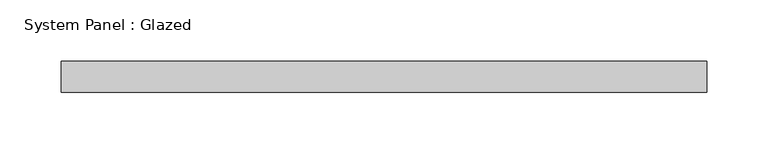
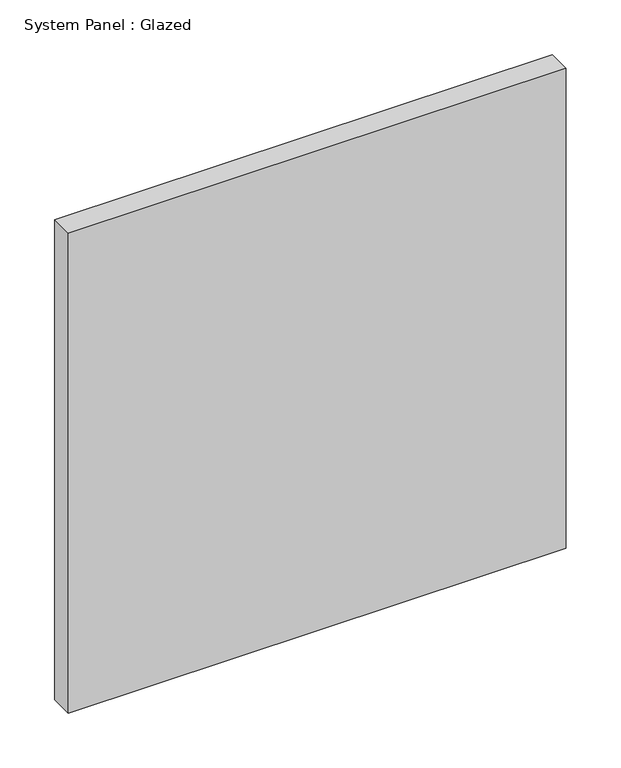
"""IFC4 building model written with IfcOpenShell, lengths in millimetres: plate geometry, System Panel : Glazed."""

from ifc_helpers import new_model, si_unit, origin, origin_with_axes, place, context, project, spatial, polyline, outline, extrude, source, transform, mapped, element, save


def system_panel_glazed_d134efab(model_context):
    return source(origin(), model_context, "Body", "SweptSolid", [
        extrude(outline(polyline([(262.5, 24.5), (-262.5, 24.5), (-262.5, 49.5), (262.5, 49.5), (262.5, 24.5)])), origin_with_axes(), (0.0, 0.0, 1.0), 535.0),
    ])


if __name__ == "__main__":
    model = new_model("IFC4")
    model_context = context("Model", 3, world=origin())
    ifc_project = project(units=[si_unit("LENGTHUNIT", "METRE", prefix="MILLI")], contexts=[model_context])
    site = spatial("IfcSite", under=ifc_project)
    building = spatial("IfcBuilding", under=site)
    placement = place(None, origin())
    system_panel_glazed_shape = system_panel_glazed_d134efab(model_context)
    element("IfcPlate", 1, ObjectType="System Panel : Glazed", at=placement, inside=building, context=model_context, shape_type="MappedRepresentation", body=[
        mapped(system_panel_glazed_shape, transform((0.0, 0.0, 0.0), x_axis=(1.0, 0.0, 0.0), y_axis=(0.0, 1.0, 0.0), z_axis=(0.0, 0.0, 1.0))),
    ])
    save(model, "model.ifc")

# Revit data of these elements
# Type "System Panel : Glazed"
#   Construction Type Id = "GSP4R"
#   Analytic Construction = "1/8 in Pilkington single glazing"
#   Visual Light Transmittance = 0.9
#   Solar Heat Gain Coefficient = 0.86
#   Heat Transfer Coefficient (U) = 6.7069 W/(m²·K)
#   Define Thermal Properties by = 1
# Element 1 (IfcPlate, "System Panel : Glazed")
#   Materials on its faces: "Glass"
# Materials
#   "Glass": class "Glass", colour RGB 0 128 192, transparency 0.9, Description = "Soda Lime Glass", Cost = 0
